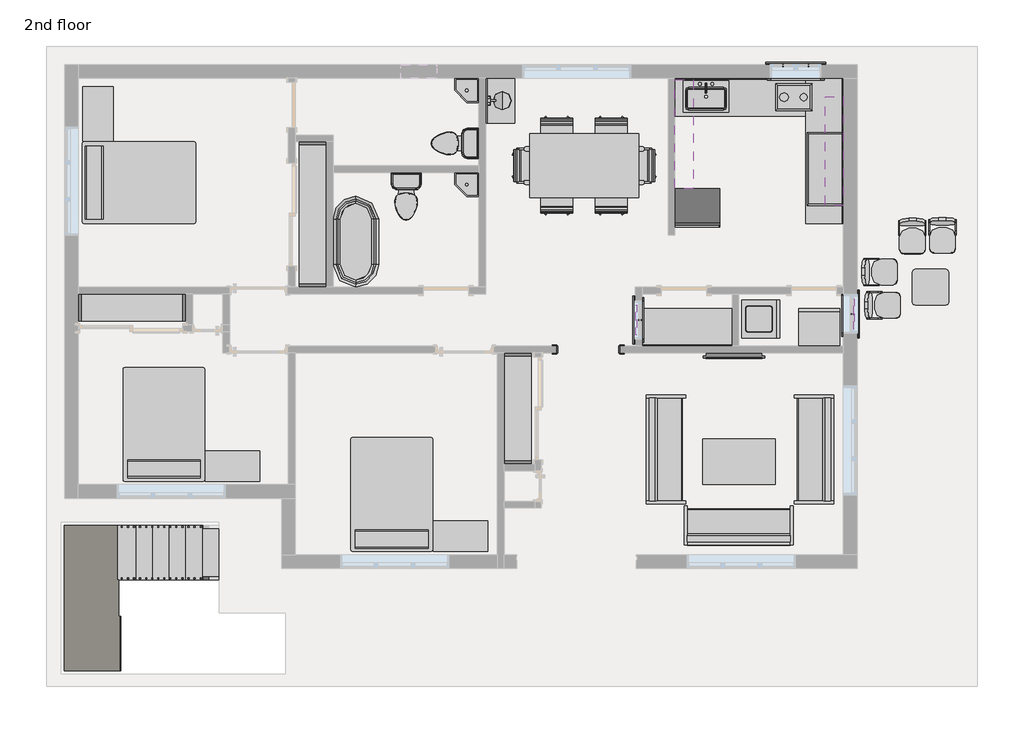
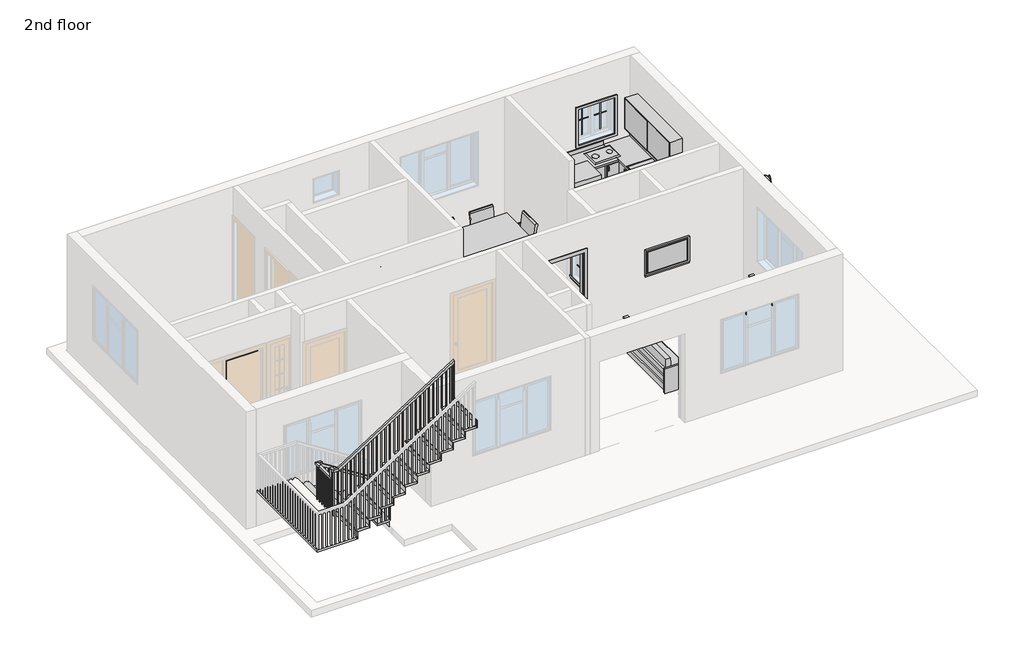
# One storey, part 4 of 4: 34 furniture elements, 17 proxies, 7 flow terminals, 2 stair flights, 1 railing, 1 slab.
# Revit data of these elements (continued)
# Type "Handrail - Rectangular" (continued)
#   built-in parameter 1008611 = 0.0416667 (stored number, unit not read)
#   built-in parameter 1008609 = 0.333333 (stored number, unit not read)
#   built-in parameter 1008604 = 0.166667 (stored number, unit not read)
#   built-in parameter 1008603 = 0.166667 (stored number, unit not read)
#   Railing Height = 3' - 0"
#   built-in parameter 1008630 = 2
#   built-in parameter 1008610 = 2
#   built-in parameter 1008618 = Baluster - Square : 3/4"
# Element 1 (IfcBuildingElementProxy, "Cook Top-2 Unit : 12\" x 18\"")
#   Phase Created = New Construction
#   Materials on its faces: "Metal - Steel, Polished", "Metal - Chrome"
# Element 2 (IfcBuildingElementProxy, "Dryer : 27\" x 25\" x 35\"")
#   Phase Created = New Construction
#   Materials on its faces: "Metal - Paint Finish - Ivory,Glossy"
# Elements 3, 4 (IfcBuildingElementProxy, "Muntin Pattern_2x2 : Muntin Pattern_2x2")
#   Width = 0' - 11 5/8"
#   Height = 2' - 6 1/2"
#   Interior Material = Wood - Stained
#   Exterior Material = Clad - White
#   Phase Created = New Construction
#   Materials on its faces: "Clad - White", "Wood - Stained"
# Elements 5, 6, 7, 8 (IfcBuildingElementProxy, "Muntin Pattern_2x2 : Muntin Pattern_2x2")
#   Width = 1' - 8"
#   Height = 1' - 5 1/8"
#   Interior Material = Wood - Stained
#   Exterior Material = Clad - White
#   Phase Created = New Construction
#   Materials on its faces: "Clad - White", "Wood - Stained"
# Element 9 (IfcBuildingElementProxy, "Passage Opening-Cased : 36\" x 84\"")
#   Phase Created = New Construction
#   Materials on its faces: "Door - Frame"
# Element 10 (IfcBuildingElementProxy, "Refrigerator-Built-in : 30\" x 24\" RH")
#   Phase Created = New Construction
#   Materials on its faces: "Metal - Paint Finish - Ivory,Glossy", "Metal - Chrome"
# Element 11 (IfcBuildingElementProxy, "Trim-Window-Exterior-Flat : with Sill")
#   Opening Width = 2' - 10"
#   Opening Height = 3' - 0"
#   Trim Material = Clad - White
#   Phase Created = New Construction
#   Materials on its faces: "Clad - White"
# Elements 12, 13 (IfcBuildingElementProxy, "Trim-Window-Exterior-Flat : with Sill")
#   Opening Width = 2' - 2"
#   Opening Height = 3' - 6"
#   Trim Material = Clad - White
#   Phase Created = New Construction
#   Materials on its faces: "Clad - White"
# Element 14 (IfcBuildingElementProxy, "Trim-Window-Interior-Flat : Picture Frame")
#   Opening Width = 2' - 10"
#   Opening Height = 3' - 0"
#   Trim Material = Wood - Stained
#   Phase Created = New Construction
#   Materials on its faces: "Wood - Stained"
# Elements 15, 16 (IfcBuildingElementProxy, "Trim-Window-Interior-Flat : Picture Frame")
#   Opening Width = 2' - 2"
#   Opening Height = 3' - 6"
#   Trim Material = Wood - Stained
#   Phase Created = New Construction
#   Materials on its faces: "Wood - Stained"
# Element 17 (IfcBuildingElementProxy, "Washer : 25\" x 25\" x 35\"")
#   Phase Created = New Construction
#   Materials on its faces: "Metal - Paint Finish - Ivory,Matte"
# Element 18 (IfcFlowTerminal, "Lavatory - Vanity : 30\"x18\" - Private")
#   Mark = "20"
#   Flow Pressure = 8.00 psi
#   Phase Created = New Construction
# Element 19 (IfcFlowTerminal, "Sink - Mop : 28\"x28\"")
#   Mark = "18"
#   Phase Created = New Construction
# Element 20 (IfcFlowTerminal, "Sink - Mop : 28\"x28\"")
#   Mark = "19"
#   Phase Created = New Construction
# Element 21 (IfcFlowTerminal, "Sink Kitchen-Single : 30\" x 21\"")
#   Mark = "17"
#   Phase Created = New Construction
#   Materials on its faces: "Steel, Polished"
# Element 22 (IfcFlowTerminal, "Toilet-Domestic-3D : Toilet-Domestic-3D")
#   Mark = "21"
#   Phase Created = New Construction
#   Materials on its faces: "Porcelain, Linen", "Laminate, Linen, Matte"
# Element 23 (IfcFlowTerminal, "Toilet-Domestic-3D : Toilet-Domestic-3D")
#   Mark = "22"
#   Phase Created = New Construction
#   Materials on its faces: "Porcelain, Linen", "Laminate, Linen, Matte"
# Element 24 (IfcFlowTerminal, "Tub-Free Standing-3D : 30\" x 60\"")
#   Mark = "16"
#   Phase Created = New Construction
#   Materials on its faces: "Porcelain, Ivory"
# Element 25 (IfcFurniture, "48\"")
#   Phase Created = New Construction
#   Materials on its faces: "Cabinets", "Cabinets - Handles"
# Element 26 (IfcFurniture, "Base Cabinet-Combo01 : 30\"")
#   Phase Created = New Construction
#   Materials on its faces: "Cabinet"
# Element 27 (IfcFurniture, "Base Cabinet-Corner Unit-Square : 36\"")
#   Phase Created = New Construction
#   Materials on its faces: "Cabinets", "Cabinets - Handles"
# Elements 28, 29, 30 (IfcFurniture, "Bed-Standard : Double 54\" x 75\"")
#   Phase Created = New Construction
#   Materials on its faces: "Linen, White", "Steel, Chrome Plated"
# Elements 31, 32, 33 (IfcFurniture, "Cabinet File-Lateral 2 Drawer : 36\" x 20\" x 24\"")
#   Phase Created = New Construction
#   Materials on its faces: "Metal - Steel"
# Elements 34, 35, 36, 37 (IfcFurniture, "Chair-Task : Chair-Task")
#   Phase Created = New Construction
#   Materials on its faces: "Plastic - Black", "Textile - Slate Blue"
# Elements 38, 39 (IfcFurniture, "Chair-Task Arms : Chair-Task Arms")
#   Phase Created = New Construction
#   Materials on its faces: "Plastic - Black", "Textile - Slate Blue"
# Element 40 (IfcFurniture, "Counter Top : 24\" Depth")
#   Length = 8' - 0"
#   Phase Created = New Construction
#   Materials on its faces: "Counter Top"
# Element 41 (IfcFurniture, "Counter Top : 24\" Depth")
#   Length = 4' - 11 1/2"
#   Phase Created = New Construction
#   Materials on its faces: "Counter Top"
# Element 42 (IfcFurniture, "Counter Top w Sink Hole : 24\" Depth")
#   Sink Opening Width = 2' - 3"
#   Sink Opening Depth = 1' - 3"
#   Sink Location To Wall = 0' - 6"
#   Sink Location = 1' - 8 1/2"
#   Length = 7' - 2 1/4"
#   Phase Created = New Construction
#   Materials on its faces: "Counter Top"
# Elements 43, 44, 45, 46 (IfcFurniture, "Seating-Auditorium : 18\" x 24\" x 30\"")
#   Phase Created = New Construction
#   Materials on its faces: "Steel, Paint Finish, Dark Gray, Matte", "Linen, Beige"
# Element 47 (IfcFurniture, "Shelving : 96\" x 12\" x 84\"")
#   Phase Created = New Construction
#   Materials on its faces: "Laminate, Ivory, Matte"
# Element 48 (IfcFurniture, "Shelving : 96\" x 12\" x 84\" 2")
#   Phase Created = New Construction
#   Materials on its faces: "Laminate, Ivory, Matte"
# Element 49 (IfcFurniture, "Shelving : 96\" x 12\" x 84\" 3")
#   Phase Created = New Construction
#   Materials on its faces: "Laminate, Ivory, Matte"
# Elements 50, 51, 52 (IfcFurniture, "Sofa : 72\"")
#   Phase Created = New Construction
#   Materials on its faces: "Cherry", "Linen, Beige"
# Element 53 (IfcFurniture, "Table-Coffee Rectangular : 48\" x 30\"")
#   Phase Created = New Construction
#   Materials on its faces: "Metal - Chrome", "Glass - Clear, Grey"
# Element 54 (IfcFurniture, "Table-Conference2 w Chairs : 40\" x 90\"")
#   Phase Created = New Construction
#   Materials on its faces: "Wood - Cherry"
# Element 55 (IfcFurniture, "Table-End : 24\" x 24\"")
#   Phase Created = New Construction
#   Materials on its faces: "Laminate, Ivory, Matte", "Birch"
# Element 56 (IfcFurniture, "Television-Plasma : 42\"")
#   Phase Created = New Construction
#   Materials on its faces: "Plastic - Gray", "Glass"
# Elements 57, 58 (IfcFurniture, "Upper Cabinet-Pass-Thru w Glass : 48\" x 30\" x 12\"")
#   Phase Created = New Construction
#   Materials on its faces: "Glass", "Cabinet"
# Element 59 (IfcRailing, "Handrail - Rectangular")
#   Phase Created = New Construction
# Element 60 (IfcSlab, "Non-Monolithic Landing")
#   Phase Created = New Construction
# Elements 61, 62 (IfcStairFlight, "2\" Tread 1\" Nosing 1/4\" Riser")
#   Phase Created = New Construction
# Materials
#   "Metal - Chrome": colour RGB 57 57 57, transparency 0
#   "Metal - Steel, Polished": colour RGB 57 57 57, transparency 0
#   "Metal - Paint Finish - Ivory,Glossy": colour RGB 247 247 239, transparency 0
#   "Door - Frame": colour RGB 118 70 51, transparency 0, Cost = 0
#   "Metal - Paint Finish - Ivory,Matte": colour RGB 247 247 239, transparency 0
#   "Steel, Polished": class "Metal", colour RGB 57 57 57, transparency 0, Description = "Polished steel", Cost = 0
#   "Porcelain, Linen": class "Ceramic", colour RGB 249 239 230, transparency 0, Description = "Porcelain, linen", Cost = 0
#   "Laminate, Linen, Matte": class "Plastic", colour RGB 249 239 230, transparency 0, Description = "Plastic Laminate - Linen, Matte", Cost = 0
#   "Porcelain, Ivory": class "Ceramic", colour RGB 247 247 239, transparency 0, Description = "Porcelain, ivory", Cost = 0
#   "Cabinets - Handles": class "Metal", colour RGB 57 57 57, transparency 0
#   "Cabinets": colour RGB 249 249 249, transparency 0
#   "Steel, Chrome Plated": class "Metal", colour RGB 17 17 17, transparency 0, Description = "Chromiuim plated steel", Cost = 0
#   "Linen, White": class "Textile", colour RGB 247 247 239, transparency 0, Description = "Linen, white", Cost = 0
#   "Metal - Steel": colour RGB 210 210 210, transparency 0
#   "Plastic - Black": colour RGB 0 0 0, transparency 0
#   "Textile - Slate Blue": colour RGB 98 102 118, transparency 0
#   "Linen, Beige": class "Textile", colour RGB 249 239 230, transparency 0, Description = "Linen, beige", Cost = 0
#   "Steel, Paint Finish, Dark Gray, Matte": class "Metal", colour RGB 0 0 0, transparency 0, Description = "Steel, paint finish, dark gray, matte", Cost = 0
#   "Laminate, Ivory, Matte": class "Plastic", colour RGB 247 247 239, transparency 0, Description = "Plastic Laminate - Ivory, Matte", Cost = 0
#   "Cherry": class "Wood", colour RGB 226 177 128, transparency 0, Description = "Prunus Serotina", Cost = 0
#   "Glass - Clear, Grey": colour RGB 252 255 255, transparency 0.64
#   "Wood - Cherry": colour RGB 151 75 0, transparency 0
#   "Birch": class "Wood", colour RGB 224 178 126, transparency 0, Description = "Betula Alleghaniensis", Cost = 0
#   "Plastic - Gray": colour RGB 134 134 134, transparency 0
#   "Clad - White": class "Wood", colour RGB 242 242 238, transparency 0, Cost = 0
#   "Wood - Stained": class "Wood", colour RGB 224 178 126, transparency 0, Cost = 0
#   "Cabinet": colour RGB 204 122 2, transparency 0
#   "Counter Top": class "Wood", colour RGB 226 177 128, transparency 0
#   "Glass": class "Glass", colour RGB 0 128 192, transparency 0.75, Description = "Soda Lime Glass", Cost = 0
